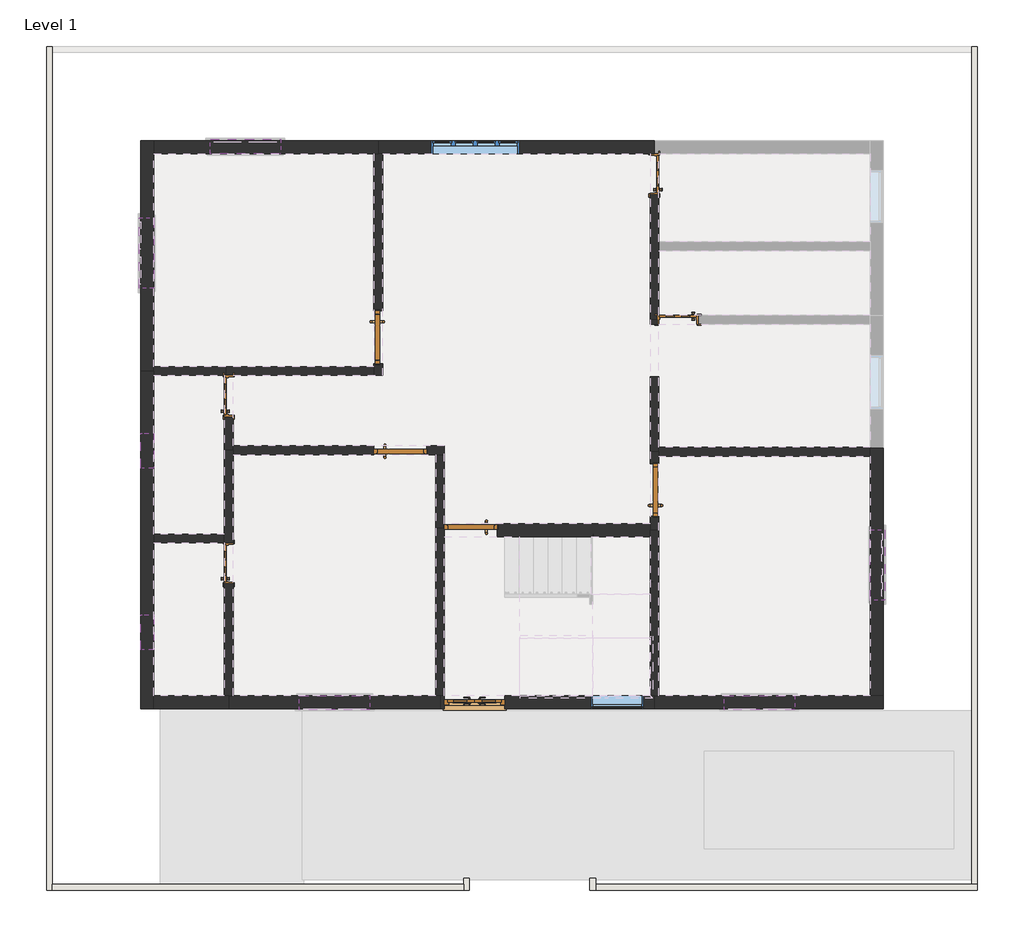
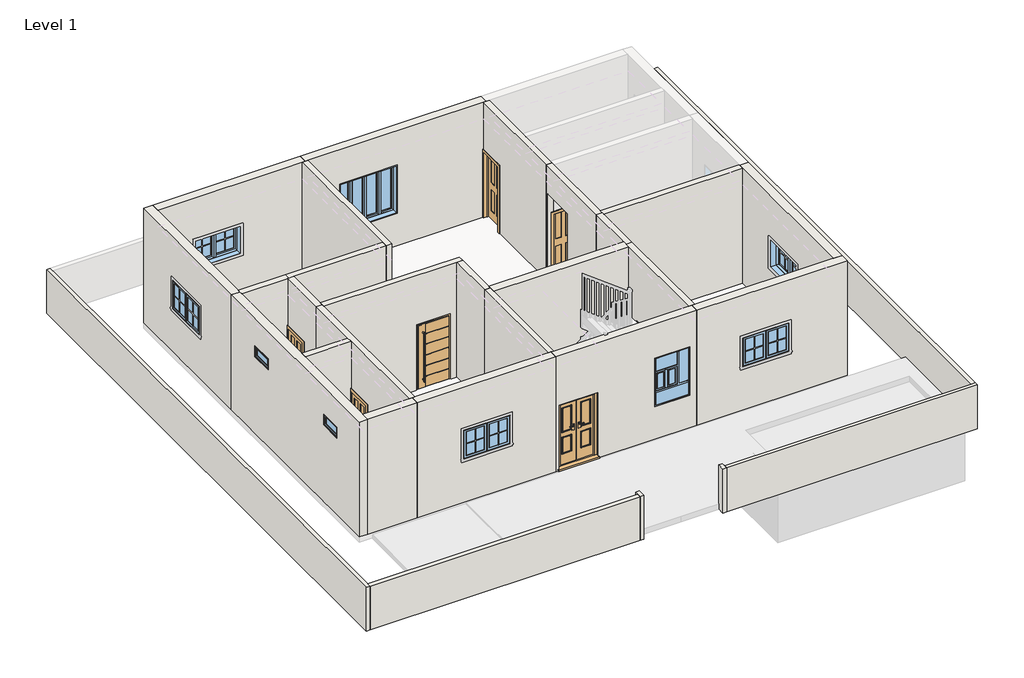
# One storey, part 1 of 2: 30 walls, 9 doors, 9 windows.
# Revit data of these elements (continued)
# Elements 18, 26 (IfcWall, "Generic - 6\"") (continued)
#   Phase Created = New Construction
#   Base Constraint = Level 1
#   Materials on its faces: "Default Wall", "BED ROOM WALL 3", "BATH ROOM WALL 1"
# Elements 19, 24 (IfcWall, "Generic - 6\"")
#   Top Offset = 0' - 0"
#   Base Offset = 0' - 0"
#   Unconnected Height = 10' - 6"
#   wall height = 10' - 6"
#   Phase Created = New Construction
#   Base Constraint = Level 1
#   Materials on its faces: "Default Wall", "BATH ROOM WALL 1"
# Element 21 (IfcWall, "Generic - 6\"")
#   Top Offset = 0' - 0"
#   Base Offset = 0' - 0"
#   Unconnected Height = 10' - 6"
#   wall height = 10' - 6"
#   Phase Created = New Construction
#   Base Constraint = Level 1
#   Materials on its faces: "Default Wall", "BED ROOM WALL 2", "LIVING"
# Element 22 (IfcWall, "Generic - 6\"")
#   Top Offset = 0' - 0"
#   Base Offset = 0' - 0"
#   Unconnected Height = 10' - 6"
#   wall height = 10' - 6"
#   Phase Created = New Construction
#   Base Constraint = Level 1
#   Materials on its faces: "Default Wall", "BED ROOM WALL 3", "LIVING 2"
# Element 25 (IfcWall, "Generic - 6\"")
#   Top Offset = 0' - 0"
#   Base Offset = 0' - 0"
#   Unconnected Height = 10' - 6"
#   wall height = 10' - 6"
#   Phase Created = New Construction
#   Base Constraint = Level 1
#   Materials on its faces: "Default Wall", "LIVING"
# Element 27 (IfcWall, "Generic - 6\"")
#   Top Offset = 0' - 0"
#   Base Offset = 0' - 0"
#   Unconnected Height = 10' - 6"
#   wall height = 10' - 6"
#   Phase Created = New Construction
#   Base Constraint = Level 1
#   Materials on its faces: "Default Wall", "BED ROOM WALL 2", "LIVING 2"
# Element 29 (IfcWall, "Generic - 6\"")
#   Top Offset = 0' - 0"
#   Base Offset = 0' - 0"
#   Unconnected Height = 10' - 6"
#   wall height = 10' - 6"
#   Phase Created = New Construction
#   Base Constraint = Level 1
#   Materials on its faces: "Default Wall", "BATH ROOM WALL 1", "LIVING"
# Elements 30, 37, 38 (IfcWall, "Generic - 9\"")
#   Top Offset = 0' - 0"
#   Base Offset = 0' - 0"
#   Unconnected Height = 10' - 6"
#   wall height = 10' - 6"
#   Phase Created = New Construction
#   Base Constraint = Level 1
#   Materials on its faces: "Default Wall", "WALL2", "BED ROOM WALL 3"
# Element 31 (IfcWall, "Generic - 9\"")
#   Top Offset = 0' - 0"
#   Base Offset = 0' - 0"
#   Unconnected Height = 10' - 6"
#   wall height = 10' - 6"
#   Phase Created = New Construction
#   Base Constraint = Level 1
#   Materials on its faces: "Default Wall", "WALL2"
# Elements 32, 34 (IfcWall, "Generic - 9\"")
#   Top Offset = 0' - 0"
#   Base Offset = 0' - 0"
#   Unconnected Height = 10' - 6"
#   wall height = 10' - 6"
#   Phase Created = New Construction
#   Base Constraint = Level 1
#   Materials on its faces: "Default Wall", "WALL2", "BED ROOM WALL 2"
# Element 33 (IfcWall, "Generic - 9\"")
#   Top Offset = 0' - 0"
#   Base Offset = 0' - 0"
#   Unconnected Height = 10' - 6"
#   wall height = 10' - 6"
#   Phase Created = New Construction
#   Base Constraint = Level 1
#   Materials on its faces: "Default Wall", "LIVING", "LIVING 2"
# Element 35 (IfcWall, "Generic - 9\"")
#   Top Offset = 0' - 0"
#   Base Offset = 0' - 0"
#   Unconnected Height = 10' - 6"
#   wall height = 10' - 6"
#   Phase Created = New Construction
#   Base Constraint = Level 1
#   Materials on its faces: "Default Wall", "WALL2", "LIVING"
# Element 36 (IfcWall, "Generic - 9\"")
#   Top Offset = 0' - 0"
#   Base Offset = 0' - 0"
#   Unconnected Height = 10' - 6"
#   wall height = 10' - 6"
#   Phase Created = New Construction
#   Base Constraint = Level 1
#   Materials on its faces: "Default Wall", "WALL2", "BATH ROOM WALL 1"
# Element 39 (IfcWall, "Generic - 9\"")
#   Top Offset = 0' - 0"
#   Base Offset = 0' - 0"
#   Unconnected Height = 10' - 6"
#   wall height = 10' - 6"
#   Phase Created = New Construction
#   Base Constraint = Level 1
#   Materials on its faces: "Default Wall", "WALL2", "LIVING 2"
# Element 40 (IfcWindow, "M_Fixed : 2'")
#   Mark = "10"
#   Phase Created = New Construction
#   Materials on its faces: "Sash", "Glass"
# Element 41 (IfcWindow, "M_Fixed : 2'")
#   Mark = "11"
#   Phase Created = New Construction
#   Materials on its faces: "Sash", "Glass"
# Element 42 (IfcWindow, "M_Window-Awning-Double-Horizontal : 4'")
#   Mark = "2"
#   Window Inset = 0' - 0"
#   Interior Wall Closure = 0' - 2.15551"
#   Frame Extension = 0' - 0 1/4"
#   Exterior Wall Closure = 0' - 1 1/4"
#   Interior Trim Visibility = yes
#   Exterior Trim Visibility = yes
#   Phase Created = New Construction
#   Materials on its faces: "Wood - Stained", "Glass", "Clad - White"
# Element 43 (IfcWindow, "M_Window-Awning-Double-Horizontal : 4'")
#   Mark = "3"
#   Window Inset = 0' - 0"
#   Interior Wall Closure = 0' - 2.15551"
#   Frame Extension = 0' - 0 1/4"
#   Exterior Wall Closure = 0' - 1 1/4"
#   Interior Trim Visibility = yes
#   Exterior Trim Visibility = yes
#   Phase Created = New Construction
#   Materials on its faces: "Wood - Stained", "Glass", "Clad - White"
# Element 44 (IfcWindow, "M_Window-Awning-Double-Horizontal : 4'")
#   Mark = "4"
#   Window Inset = 0' - 0"
#   Interior Wall Closure = 0' - 2.15551"
#   Frame Extension = 0' - 0 1/4"
#   Exterior Wall Closure = 0' - 1 1/4"
#   Interior Trim Visibility = yes
#   Exterior Trim Visibility = yes
#   Phase Created = New Construction
#   Materials on its faces: "Wood - Stained", "Glass", "Clad - White"
# Element 45 (IfcWindow, "M_Window-Awning-Double-Horizontal : 4'")
#   Mark = "5"
#   Window Inset = 0' - 0"
#   Interior Wall Closure = 0' - 2.15551"
#   Frame Extension = 0' - 0 1/4"
#   Exterior Wall Closure = 0' - 1 1/4"
#   Interior Trim Visibility = yes
#   Exterior Trim Visibility = yes
#   Phase Created = New Construction
#   Materials on its faces: "Wood - Stained", "Glass", "Clad - White"
# Element 46 (IfcWindow, "M_Window-Awning-Double-Horizontal : 4'")
#   Mark = "1"
#   Window Inset = 0' - 0"
#   Interior Wall Closure = 0' - 2.15551"
#   Frame Extension = 0' - 0 1/4"
#   Exterior Wall Closure = 0' - 1 1/4"
#   Interior Trim Visibility = yes
#   Exterior Trim Visibility = yes
#   Phase Created = New Construction
#   Materials on its faces: "Wood - Stained", "Glass", "Clad - White"
# Element 47 (IfcWindow, "M_Window-Casement-Double-Sash-Variable : 3'")
#   Mark = "9"
#   Window Inset = 0' - 0 5/8"
#   Frame Gap 3 = 0' - 1.65041"
#   Frame Gap 2 = 0' - 0.62598"
#   Phase Created = New Construction
#   Materials on its faces: "Metal - Aluminum", "Glass"
# Element 48 (IfcWindow, "M_Window-Casement-Multi-Sash-Horizontal : 5'")
#   Mark = "6"
#   Window Inset = 0' - 0.62598"
#   Frame Gap 3 = 0' - 1.62992"
#   Frame Gap 2 = 0' - 0.62598"
#   Phase Created = New Construction
#   Materials on its faces: "Metal - Aluminum", "Glass"
# Materials
#   "Door - Glazing": colour RGB 0 0 255, transparency 0.75
#   "Door - Panel": class "Wood", colour RGB 210 159 95, transparency 0, Cost = 0
#   "Door - Handle": colour RGB 0 0 0, transparency 0, Cost = 0
#   "Cherry": class "Wood", colour RGB 226 177 128, transparency 0, Description = "Prunus Serotina", Cost = 0
#   "Aluminum": class "Metal", colour RGB 247 247 247, transparency 0, Description = "Aluminum 6061", Cost = 0
#   "Sash": class "Wood", colour RGB 224 178 126, transparency 0, Cost = 0
#   "Glass": class "Glass", colour RGB 0 128 192, transparency 0.9, Description = "Soda Lime Glass", Cost = 0
#   "Wood - Stained": class "Wood", colour RGB 224 178 126, transparency 0, Cost = 0
#   "Clad - White": class "Wood", colour RGB 242 242 238, transparency 0, Cost = 0
#   "Metal - Aluminum": class "Metal", colour RGB 247 247 247, transparency 0
#   "Default Wall": colour RGB 128 128 128, transparency 0, Cost = 0
#   "LIVING": class "Generic", colour RGB 120 120 120, transparency 0, Cost = 0
#   "BED ROOM WALL 2": class "Generic", colour RGB 120 120 120, transparency 0, Cost = 0
#   "BED ROOM WALL 3": class "Generic", colour RGB 120 120 120, transparency 0, Cost = 0
#   "BATH ROOM WALL 1": class "Generic", colour RGB 120 120 120, transparency 0, Cost = 0
#   "LIVING 2": class "Generic", colour RGB 120 120 120, transparency 0, Cost = 0
#   "WALL2": class "Generic", colour RGB 120 120 120, transparency 0, Cost = 0
